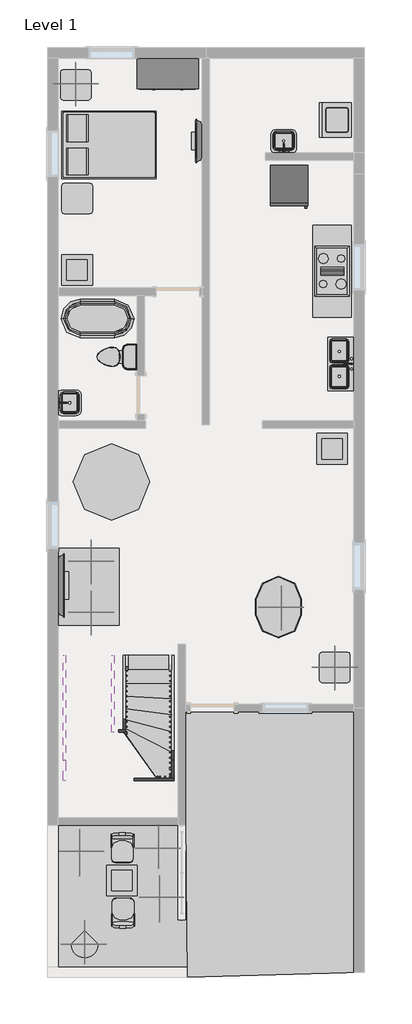
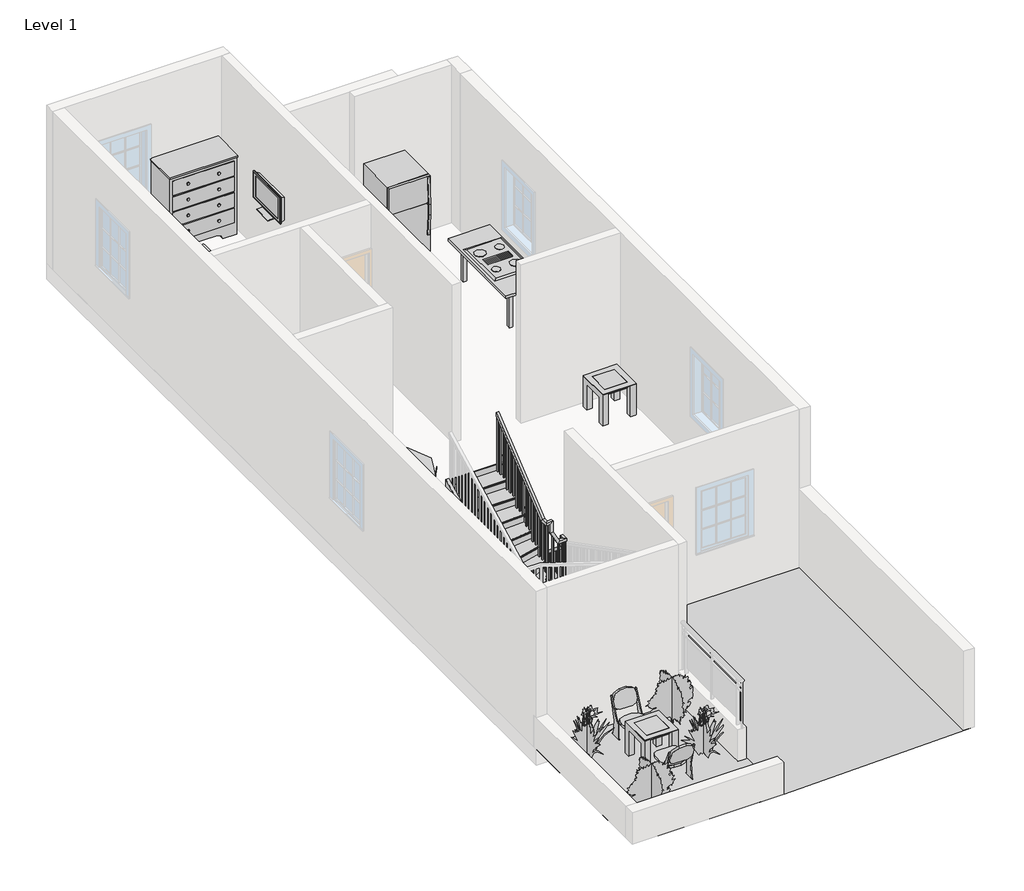
# One storey, part 3 of 3: 16 furniture elements, 9 geographic elements, 8 members, 7 flow terminals, 5 proxies, 1 railing, 1 stair flight.
"""IFC4 building model written with IfcOpenShell, lengths in millimetres."""

from ifc_helpers import new_model, si_unit, frame, origin, place, context, project, spatial, polyline, outline, extrude, faceted_brep, triangles, transform, mapped, element, save
from components import proxy_bb1e6e30, proxy_a13a33b2, proxy_718fa39f, flow_terminal_2b63360b, flow_terminal_a53be723, flow_terminal_62a433f7, toilet_domestic_3d_toilet_domestic_3d_f7549cf7, toilet_domestic_3d_toilet_domestic_3d_183bbd19, flow_terminal_db991eef, furniture_c8abb964, furniture_2babcf72, furniture_3d1d9cbc, furniture_56245f3a, furniture_fdf74506, furniture_b5c51a22, furniture_be1c6672, furniture_bbcc68ce, furniture_31d08a24, furniture_e8434c74, furniture_a5b052b6, rpc_plant_tropical_55f6ff97, rpc_plant_tropical_agave_1_5_93a2a214, rpc_plant_tropical_jungle_flame_3_9c4808c2, stair_flight_35bc4011

model = new_model("IFC4")

# Units and contexts
model_context = context("Model", 3, world=origin())
ifc_project = project(units=[si_unit("LENGTHUNIT", "METRE", prefix="MILLI")], contexts=[model_context])

# Site, building, storey
site = spatial("IfcSite", under=ifc_project)
building = spatial("IfcBuilding", under=site)
storey = spatial("IfcBuildingStorey", under=building, Name="Level 1", Elevation=0.0)

# Proxies
placement = place(None, origin())
element("IfcBuildingElementProxy", 1, Name="Building Element Proxy", at=placement, inside=storey, context=model_context, shape_type="Tessellation", body=[
    triangles([(-3017.7480675, -2501.1894814, 0.0), (-3017.7480675, -5523.7895782, 0.0), (-249.1479645, -5523.7895782, 0.0), (-274.5479585, -2501.1894814, 0.0)], [[1, 2, 4], [3, 4, 2]], closed=False),
])
element("IfcBuildingElementProxy", 2, Name="Building Element Proxy", at=placement, inside=storey, context=model_context, shape_type="Tessellation", body=[
    triangles([(-274.5479585, -240.5896025, 0.0), (3281.4520294, -240.5896025, 0.0), (3281.4520294, -5422.1893845, 0.0), (-249.1479645, -5523.7895782, 0.0), (-172.9479645, -138.9895994, 0.0)], [[1, 4, 3], [1, 2, 5], [2, 1, 3]], closed=False),
])
proxy_shape = proxy_bb1e6e30(model_context)
element("IfcBuildingElementProxy", 3, Name="Cook Top-4 Unit : 36\" x 20\"", ObjectType="Cook Top-4 Unit : 36\" x 20\"", at=placement, inside=storey, context=model_context, shape_type="MappedRepresentation", body=[
    mapped(proxy_shape, transform((2646.4520363, 8522.4104001, 0.0), x_axis=(0.0, -1.0, 0.0), y_axis=(1.0, 0.0, 0.0), z_axis=(0.0, 0.0, 1.0))),
])
proxy_2_shape = proxy_a13a33b2(model_context)
element("IfcBuildingElementProxy", 4, Name="Refrigerator : 30\" x 32\" RH", ObjectType="Refrigerator : 30\" x 32\" RH", at=placement, inside=storey, context=model_context, shape_type="MappedRepresentation", body=[
    mapped(proxy_2_shape, transform((1790.7895363, 10242.0614286, 0.0), x_axis=(1.0, 0.0, 0.0), y_axis=(0.0, 1.0, 0.0), z_axis=(0.0, 0.0, 1.0))),
])
proxy_3_shape = proxy_718fa39f(model_context)
element("IfcBuildingElementProxy", 5, Name="Washer : 27\" x 25\" x 35\"", ObjectType="Washer : 27\" x 25\" x 35\"", at=placement, inside=storey, context=model_context, shape_type="MappedRepresentation", body=[
    mapped(proxy_3_shape, transform((2989.1016011, 11111.8929316, 0.0), x_axis=(0.0, 1.0000000000000007, 0.0), y_axis=(-1.0000000000000007, 0.0, 0.0), z_axis=(0.0, 0.0, 1.0))),
])

# Flow terminals
flow_terminal_shape = flow_terminal_2b63360b(model_context)
element("IfcFlowTerminal", 6, ObjectType="Floor Drain - Rectangular : 5\"x5\" Strainer - 2\" Drain", at=placement, inside=storey, context=model_context, shape_type="MappedRepresentation", body=[
    mapped(flow_terminal_shape, transform((-2636.7479637, 7100.0104001, 0.0), x_axis=(1.0, 0.0, 0.0), y_axis=(0.0, 1.0, 0.0), z_axis=(0.0, 0.0, 1.0))),
])
element("IfcFlowTerminal", 7, ObjectType="Floor Drain - Rectangular : 5\"x5\" Strainer - 2\" Drain", at=placement, inside=storey, context=model_context, shape_type="MappedRepresentation", body=[
    mapped(flow_terminal_shape, transform((2849.6520363, 12205.4104001, 0.0), x_axis=(1.0, 0.0, 0.0), y_axis=(0.0, 1.0, 0.0), z_axis=(0.0, 0.0, 1.0))),
])
flow_terminal_2_shape = flow_terminal_a53be723(model_context)
element("IfcFlowTerminal", 8, ObjectType="Sink Kitchen-Double : 42\" x 21\"", at=placement, inside=storey, context=model_context, shape_type="MappedRepresentation", body=[
    mapped(flow_terminal_2_shape, transform((2821.9066352, 6696.5996407, 0.0), x_axis=(0.0, -1.0000000000000004, 0.0), y_axis=(1.0000000000000004, 0.0, 0.0), z_axis=(0.0, 0.0, 1.0))),
])
flow_terminal_3_shape = flow_terminal_62a433f7(model_context)
element("IfcFlowTerminal", 9, ObjectType="Sink Vanity-Square : 20\" x 18\"", at=placement, inside=storey, context=model_context, shape_type="MappedRepresentation", body=[
    mapped(flow_terminal_3_shape, transform((-2634.4025626, 5890.5211595, 0.0), x_axis=(0.0, 1.0000000000000002, 0.0), y_axis=(-1.0000000000000002, 0.0, 0.0), z_axis=(0.0, 0.0, 1.0))),
])
element("IfcFlowTerminal", 10, ObjectType="Sink Vanity-Square : 20\" x 18\"", at=placement, inside=storey, context=model_context, shape_type="MappedRepresentation", body=[
    mapped(flow_terminal_3_shape, transform((1696.9412769, 11064.7558012, 0.0), x_axis=(-1.0000000000000004, 0.0, 0.0), y_axis=(0.0, -1.0000000000000004, 0.0), z_axis=(0.0, 0.0, 1.0))),
])
toilet_domestic_3d_toilet_domestic_3d_shape = toilet_domestic_3d_toilet_domestic_3d_f7549cf7(model_context)
toilet_domestic_3d_toilet_domestic_3d_2_shape = toilet_domestic_3d_toilet_domestic_3d_183bbd19(model_context)
element("IfcFlowTerminal", 11, ObjectType="Toilet-Domestic-3D : Toilet-Domestic-3D", at=placement, inside=storey, context=model_context, shape_type="MappedRepresentation", body=[
    mapped(toilet_domestic_3d_toilet_domestic_3d_shape, transform((-1734.443991, 6820.6104001, 0.0), x_axis=(0.0, -1.0000000000000004, 0.0), y_axis=(1.0000000000000004, 0.0, 0.0), z_axis=(0.0, 0.0, 1.0))),
    mapped(toilet_domestic_3d_toilet_domestic_3d_2_shape, transform((-1734.443991, 6820.6104001, 0.0), x_axis=(0.0, -1.0000000000000004, 0.0), y_axis=(1.0000000000000004, 0.0, 0.0), z_axis=(0.0, 0.0, 1.0))),
])
flow_terminal_4_shape = flow_terminal_db991eef(model_context)
element("IfcFlowTerminal", 12, ObjectType="Tub-Free Standing-3D : 30\" x 60\"", at=placement, inside=storey, context=model_context, shape_type="MappedRepresentation", body=[
    mapped(flow_terminal_4_shape, transform((-2027.1479637, 7582.6104001, 0.0), x_axis=(0.0, 1.0000000000000002, 0.0), y_axis=(-1.0000000000000002, 0.0, 0.0), z_axis=(0.0, 0.0, 1.0))),
])

# Furniture
furniture_shape = furniture_c8abb964(model_context)
element("IfcFurniture", 13, ObjectType="Bed-Box : Double 53\" x 74\"", at=placement, inside=storey, context=model_context, shape_type="MappedRepresentation", body=[
    mapped(furniture_shape, transform((-2032.9774719, 10697.8579411, 0.0), x_axis=(0.0, 1.0, 0.0), y_axis=(-1.0, 0.0, 0.0), z_axis=(0.0, 0.0, 1.0))),
])
furniture_2_shape = furniture_2babcf72(model_context)
element("IfcFurniture", 14, ObjectType="Dresser : 48\" x 60\" x 24\"", at=placement, inside=storey, context=model_context, shape_type="MappedRepresentation", body=[
    mapped(furniture_2_shape, transform((-360.9547039, 12822.5733542, 0.0), x_axis=(1.0, 0.0, 0.0), y_axis=(0.0, 1.0, 0.0), z_axis=(0.0, 0.0, 1.0))),
])
furniture_3_shape = furniture_3d1d9cbc(model_context)
element("IfcFurniture", 15, ObjectType="Seating-Auditorium : 18\" x 24\" x 30\"", at=placement, inside=storey, context=model_context, shape_type="MappedRepresentation", body=[
    mapped(furniture_3_shape, transform((-1371.1200948, -2743.1141901, 0.0), x_axis=(-1.0000000000000004, 0.0, 0.0), y_axis=(0.0, -1.0000000000000004, 0.0), z_axis=(0.0, 0.0, 1.0))),
])
element("IfcFurniture", 16, ObjectType="Seating-Auditorium : 18\" x 24\" x 30\"", at=placement, inside=storey, context=model_context, shape_type="MappedRepresentation", body=[
    mapped(furniture_3_shape, transform((-1679.8758325, -4443.6650097, 0.0), x_axis=(1.0, 0.0, 0.0), y_axis=(0.0, 1.0, 0.0), z_axis=(0.0, 0.0, 1.0))),
])
furniture_4_shape = furniture_56245f3a(model_context)
element("IfcFurniture", 17, ObjectType="TV - Flat Screen : 32\"", at=placement, inside=storey, context=model_context, shape_type="MappedRepresentation", body=[
    mapped(furniture_4_shape, transform((-2.8865873, 11109.265886, 1041.4), x_axis=(0.0, -1.0000000000000002, 0.0), y_axis=(1.0000000000000002, 0.0, 0.0), z_axis=(0.0, 0.0, 1.0))),
])
furniture_5_shape = furniture_fdf74506(model_context)
element("IfcFurniture", 18, ObjectType="TV - Flat Screen : 50\"", at=placement, inside=storey, context=model_context, shape_type="MappedRepresentation", body=[
    mapped(furniture_5_shape, transform((-2756.00934, 2277.9549142, 1041.4), x_axis=(0.0, 1.0000000000000002, 0.0), y_axis=(-1.0000000000000002, 0.0, 0.0), z_axis=(0.0, 0.0, 1.0))),
])
furniture_6_shape = furniture_b5c51a22(model_context)
element("IfcFurniture", 19, ObjectType="Table-Coffee : 24\" x 24\" x 24\"", at=placement, inside=storey, context=model_context, shape_type="MappedRepresentation", body=[
    mapped(furniture_6_shape, transform((-2451.8137304, 8452.5993223, 0.0), x_axis=(1.0, 0.0, 0.0), y_axis=(0.0, 1.0, 0.0), z_axis=(0.0, 0.0, 1.0))),
])
element("IfcFurniture", 20, ObjectType="Table-Coffee : 24\" x 24\" x 24\"", at=placement, inside=storey, context=model_context, shape_type="MappedRepresentation", body=[
    mapped(furniture_6_shape, transform((2628.1862696, 4896.5993223, 0.0), x_axis=(1.0, 0.0, 0.0), y_axis=(0.0, 1.0, 0.0), z_axis=(0.0, 0.0, 1.0))),
])
element("IfcFurniture", 21, ObjectType="Table-Coffee : 24\" x 24\" x 24\"", at=placement, inside=storey, context=model_context, shape_type="MappedRepresentation", body=[
    mapped(furniture_6_shape, transform((-1562.8137304, -3688.6006777, 0.0), x_axis=(1.0, 0.0, 0.0), y_axis=(0.0, 1.0, 0.0), z_axis=(0.0, 0.0, 1.0))),
])
furniture_7_shape = furniture_be1c6672(model_context)
element("IfcFurniture", 22, ObjectType="Table-Dining Oval : 36\" x 48\"", at=placement, inside=storey, context=model_context, shape_type="MappedRepresentation", body=[
    mapped(furniture_7_shape, transform((1221.5536757, 2244.0300722, 0.0), x_axis=(0.0, 1.0000000000000002, 0.0), y_axis=(-1.0000000000000002, 0.0, 0.0), z_axis=(0.0, 0.0, 1.0))),
])
furniture_8_shape = furniture_bbcc68ce(model_context)
element("IfcFurniture", 23, ObjectType="Table-Dining Round w Chairs : 60\" Diameter", at=placement, inside=storey, context=model_context, shape_type="MappedRepresentation", body=[
    mapped(furniture_8_shape, transform((-1851.4299309, 4516.2890886, 0.0), x_axis=(1.0, 0.0, 0.0), y_axis=(0.0, 1.0, 0.0), z_axis=(0.0, 0.0, 1.0))),
])
furniture_9_shape = furniture_31d08a24(model_context)
element("IfcFurniture", 24, ObjectType="Table-End : 24\" x 24\"", at=placement, inside=storey, context=model_context, shape_type="MappedRepresentation", body=[
    mapped(furniture_9_shape, transform((-2767.481594, 12078.4104001, 0.0), x_axis=(1.0, 0.0, 0.0), y_axis=(0.0, 1.0, 0.0), z_axis=(0.0, 0.0, 1.0))),
])
element("IfcFurniture", 25, ObjectType="Table-End : 24\" x 24\"", at=placement, inside=storey, context=model_context, shape_type="MappedRepresentation", body=[
    mapped(furniture_9_shape, transform((-2742.081594, 9817.8104001, 0.0), x_axis=(1.0, 0.0, 0.0), y_axis=(0.0, 1.0, 0.0), z_axis=(0.0, 0.0, 1.0))),
])
element("IfcFurniture", 26, ObjectType="Table-End : 24\" x 24\"", at=placement, inside=storey, context=model_context, shape_type="MappedRepresentation", body=[
    mapped(furniture_9_shape, transform((2388.718406, 492.2787082, 0.0), x_axis=(1.0, 0.0, 0.0), y_axis=(0.0, 1.0, 0.0), z_axis=(0.0, 0.0, 1.0))),
])
furniture_10_shape = furniture_e8434c74(model_context)
element("IfcFurniture", 27, ObjectType="Table-Rectangular : 60\" x 48\"", at=placement, inside=storey, context=model_context, shape_type="MappedRepresentation", body=[
    mapped(furniture_10_shape, transform((-2204.9479637, 2248.6104001, 0.0), x_axis=(0.0, 1.0, 0.0), y_axis=(-1.0, 0.0, 0.0), z_axis=(0.0, 0.0, 1.0))),
])
furniture_11_shape = furniture_a5b052b6(model_context)
element("IfcFurniture", 28, ObjectType="Table-Rectangular : 72\" x 30\"", at=placement, inside=storey, context=model_context, shape_type="MappedRepresentation", body=[
    mapped(furniture_11_shape, transform((2646.4520363, 8522.4104001, 0.0), x_axis=(0.0, 1.0, 0.0), y_axis=(-1.0, 0.0, 0.0), z_axis=(0.0, 0.0, 1.0))),
])

# Geographic elements
rpc_plant_tropical_shape = rpc_plant_tropical_55f6ff97(model_context)
element("IfcGeographicElement", 29, ObjectType="RPC Plant - Tropical", at=placement, inside=storey, context=model_context, shape_type="MappedRepresentation", body=[
    mapped(rpc_plant_tropical_shape, transform((-2382.7479637, -3009.1895999, 0.0), x_axis=(1.0, 0.0, 0.0), y_axis=(0.0, 1.0, 0.0), z_axis=(0.0, 0.0, 1.0))),
])
element("IfcGeographicElement", 30, ObjectType="RPC Plant - Tropical", at=placement, inside=storey, context=model_context, shape_type="MappedRepresentation", body=[
    mapped(rpc_plant_tropical_shape, transform((-788.8979637, -3923.5895999, 0.0), x_axis=(1.0, 0.0, 0.0), y_axis=(0.0, 1.0, 0.0), z_axis=(0.0, 0.0, 1.0))),
])
rpc_plant_tropical_agave_1_5_shape = rpc_plant_tropical_agave_1_5_93a2a214(model_context)
element("IfcGeographicElement", 31, ObjectType="RPC Plant - Tropical : Agave - 1.5'", at=placement, inside=storey, context=model_context, shape_type="MappedRepresentation", body=[
    mapped(rpc_plant_tropical_agave_1_5_shape, transform((-2458.9479637, 12256.2104001, 609.6), x_axis=(1.0, 0.0, 0.0), y_axis=(0.0, 1.0, 0.0), z_axis=(0.0, 0.0, 1.0))),
])
element("IfcGeographicElement", 32, ObjectType="RPC Plant - Tropical : Agave - 1.5'", at=placement, inside=storey, context=model_context, shape_type="MappedRepresentation", body=[
    mapped(rpc_plant_tropical_agave_1_5_shape, transform((2697.2520363, 644.6787082, 609.6), x_axis=(1.0, 0.0, 0.0), y_axis=(0.0, 1.0, 0.0), z_axis=(0.0, 0.0, 1.0))),
])
element("IfcGeographicElement", 33, ObjectType="RPC Plant - Tropical : Agave - 1.5'", at=placement, inside=storey, context=model_context, shape_type="MappedRepresentation", body=[
    mapped(rpc_plant_tropical_agave_1_5_shape, transform((1630.4520363, 1842.2104001, 609.6), x_axis=(1.0, 0.0, 0.0), y_axis=(0.0, 1.0, 0.0), z_axis=(0.0, 0.0, 1.0))),
])
element("IfcGeographicElement", 34, ObjectType="RPC Plant - Tropical : Agave - 1.5'", at=placement, inside=storey, context=model_context, shape_type="MappedRepresentation", body=[
    mapped(rpc_plant_tropical_agave_1_5_shape, transform((-2154.1479637, 2756.6104001, 660.4), x_axis=(1.0, 0.0, 0.0), y_axis=(0.0, 1.0, 0.0), z_axis=(0.0, 0.0, 1.0))),
])
element("IfcGeographicElement", 35, ObjectType="RPC Plant - Tropical : Agave - 1.5'", at=placement, inside=storey, context=model_context, shape_type="MappedRepresentation", body=[
    mapped(rpc_plant_tropical_agave_1_5_shape, transform((-2154.1479637, 1740.6104001, 660.4), x_axis=(1.0, 0.0, 0.0), y_axis=(0.0, 1.0, 0.0), z_axis=(0.0, 0.0, 1.0))),
])
rpc_plant_tropical_jungle_flame_3_shape = rpc_plant_tropical_jungle_flame_3_9c4808c2(model_context)
element("IfcGeographicElement", 36, ObjectType="RPC Plant - Tropical : Jungle Flame - 3'", at=placement, inside=storey, context=model_context, shape_type="MappedRepresentation", body=[
    mapped(rpc_plant_tropical_jungle_flame_3_shape, transform((-2281.1479637, -4863.3895999, 0.0), x_axis=(1.0, 0.0, 0.0), y_axis=(0.0, 1.0, 0.0), z_axis=(0.0, 0.0, 1.0))),
])
element("IfcGeographicElement", 37, ObjectType="RPC Plant - Tropical : Jungle Flame - 3'", at=placement, inside=storey, context=model_context, shape_type="MappedRepresentation", body=[
    mapped(rpc_plant_tropical_jungle_flame_3_shape, transform((-807.9479637, -2958.3895999, 0.0), x_axis=(1.0, 0.0, 0.0), y_axis=(0.0, 1.0, 0.0), z_axis=(0.0, 0.0, 1.0))),
])

# Members
element("IfcMember", 38, ObjectType="Stringer - 2\" Width", at=placement, inside=storey, context=model_context, shape_type="SweptSolid", body=[
    extrude(outline(polyline([(880.742092, 229.639954), (880.742092, 0.0), (660.9797744, 0.0), (-1206.6750997, 962.500629), (-1206.6750997, 1305.3956453), (880.742092, 229.639954)])), frame((-553.9479637, 0.0, 0.0), z_axis=(1.0, 0.0, 0.0), x_axis=(0.0, 1.0, 0.0)), (0.0, 0.0, 1.0), 50.8),
])
element("IfcMember", 39, ObjectType="Stringer - 2\" Width", at=placement, inside=storey, context=model_context, shape_type="SweptSolid", body=[
    extrude(outline(polyline([(-553.9479637, -1206.6750997), (-503.1479637, -1206.6750997), (-503.1479637, -1561.3895999), (-553.9479637, -1561.3895999), (-553.9479637, -1206.6750997)])), frame((0.0, 0.0, 962.500629), z_axis=(0.0, 0.0, 1.0), x_axis=(1.0, 0.0, 0.0)), (0.0, 0.0, 1.0), 342.8950162),
])
element("IfcMember", 40, ObjectType="Stringer - 2\" Width", at=placement, inside=storey, context=model_context, shape_type="SweptSolid", body=[
    extrude(outline(polyline([(1000.5956453, -503.1479637), (1289.0952212, -503.1479637), (1969.9972697, -2625.1678464), (1969.9972697, -2662.1479637), (1638.9682298, -2662.1479637), (1000.5956453, -672.6704467), (1000.5956453, -503.1479637)])), frame((0.0, -1612.1895999, 0.0), z_axis=(0.0, 1.0, 0.0), x_axis=(0.0, 0.0, 1.0)), (0.0, 0.0, 1.0), 50.8),
])
element("IfcMember", 41, ObjectType="Stringer - 2\" Width", at=placement, inside=storey, context=model_context, shape_type="SweptSolid", body=[
    extrude(outline(polyline([(-2662.1479637, -1612.1895999), (-2712.9479637, -1612.1895999), (-2712.9479637, -1206.6750997), (-2662.1479637, -1206.6750997), (-2662.1479637, -1612.1895999)])), frame((0.0, 0.0, 1649.8904473), z_axis=(0.0, 0.0, 1.0), x_axis=(1.0, 0.0, 0.0)), (0.0, 0.0, 1.0), 320.1068224),
])
element("IfcMember", 42, ObjectType="Stringer - 2\" Width", at=placement, inside=storey, context=model_context, shape_type="SweptSolid", body=[
    extrude(outline(polyline([(-1206.6750997, 1649.8904473), (-1206.6750997, 1969.9972697), (880.742092, 3045.7529609), (880.742092, 2725.6461385), (-1206.6750997, 1649.8904473)])), frame((-2712.9479637, 0.0, 0.0), z_axis=(1.0, 0.0, 0.0), x_axis=(0.0, 1.0, 0.0)), (0.0, 0.0, 1.0), 50.8),
])
element("IfcMember", 43, ObjectType="Stringer - 2\" Width", at=placement, inside=storey, context=model_context, shape_type="SweptSolid", body=[
    extrude(outline(polyline([(880.742092, 176.1764461), (880.742092, 0.0), (614.4804474, 0.0), (-596.1895999, 987.1410923), (-596.1895999, 1380.418648), (880.742092, 176.1764461)])), frame((-1519.1479637, 0.0, 0.0), z_axis=(1.0, 0.0, 0.0), x_axis=(0.0, 1.0, 0.0)), (0.0, 0.0, 1.0), 50.8),
])
element("IfcMember", 44, ObjectType="Stringer - 2\" Width", at=placement, inside=storey, context=model_context, shape_type="SweptSolid", body=[
    extrude(outline(polyline([(1028.5617647, -1468.3479637), (1573.2682978, -1468.3479637), (1926.1409689, -1674.9850811), (1926.1409689, -1696.9479637), (1360.465107, -1696.9479637), (1028.5617647, -1502.590181), (1028.5617647, -1468.3479637)])), frame((0.0, -646.9895999, 0.0), z_axis=(0.0, 1.0, 0.0), x_axis=(0.0, 0.0, 1.0)), (0.0, 0.0, 1.0), 50.8),
])
element("IfcMember", 45, ObjectType="Stringer - 2\" Width", at=placement, inside=storey, context=model_context, shape_type="SweptSolid", body=[
    extrude(outline(polyline([(-646.9895999, 1532.8634131), (-646.9895999, 1926.1409689), (880.742092, 3171.8038432), (880.742092, 2778.5262875), (-646.9895999, 1532.8634131)])), frame((-1747.7479637, 0.0, 0.0), z_axis=(1.0, 0.0, 0.0), x_axis=(0.0, 1.0, 0.0)), (0.0, 0.0, 1.0), 50.8),
])

# Railing
element("IfcRailing", 46, ObjectType="Handrail - Rectangular", at=placement, inside=storey, context=model_context, shape_type="SolidModel", body=[
    faceted_brep([(-1417.5479637, 880.742092, 1025.2529681), (-1417.5479637, 880.742092, 959.7067088), (-1468.3479637, 880.742092, 959.7067088), (-1468.3479637, 880.742092, 1025.2529681), (-1417.5479637, -570.7895999, 2208.7848338), (-1417.5479637, -621.5895999, 2184.659247), (-1468.3479637, -621.5895999, 2184.659247), (-1468.3479637, -570.7895999, 2208.7848338), (-1417.5479637, -570.7895999, 2414.6281882), (-1417.5479637, -621.5895999, 2363.8281882), (-1468.3479637, -621.5895999, 2363.8281882), (-1468.3479637, -570.7895999, 2414.6281882), (-1417.5479637, -697.7895999, 2414.6281882), (-1417.5479637, -697.7895999, 2363.8281882), (-1468.3479637, -646.9895999, 2363.8281882), (-1468.3479637, -646.9895999, 2414.6281882), (-1544.5479637, -697.7895999, 2414.6281882), (-1573.6692975, -697.7895999, 2363.8281882), (-1573.6692975, -646.9895999, 2363.8281882), (-1544.5479637, -646.9895999, 2414.6281882), (-1671.5479637, -697.7895999, 2631.5051451), (-1722.3479637, -697.7895999, 2617.7256424), (-1722.3479637, -646.9895999, 2617.7256424), (-1671.5479637, -646.9895999, 2631.5051451), (-1671.5479637, -697.7895999, 2837.3484995), (-1722.3479637, -697.7895999, 2786.5484995), (-1722.3479637, -646.9895999, 2786.5484995), (-1671.5479637, -646.9895999, 2837.3484995), (-1798.5479637, -697.7895999, 2837.3484995), (-1798.5479637, -697.7895999, 2786.5484995), (-1747.7479637, -646.9895999, 2786.5484995), (-1747.7479637, -646.9895999, 2837.3484995), (-1798.5479637, -570.7895999, 2837.3484995), (-1798.5479637, -552.7041868, 2786.5484995), (-1747.7479637, -552.7041868, 2786.5484995), (-1747.7479637, -570.7895999, 2837.3484995), (-1798.5479637, 880.742092, 4020.8803652), (-1747.7479637, 880.742092, 4020.8803652), (-1747.7479637, 880.742092, 3955.3341059), (-1798.5479637, 880.742092, 3955.3341059)], [[[0, 1, 2, 3]], [[1, 0, 4, 5]], [[2, 1, 5, 6]], [[3, 2, 6, 7]], [[0, 3, 7, 4]], [[5, 4, 8, 9]], [[6, 5, 9, 10]], [[7, 6, 10, 11]], [[4, 7, 11, 8]], [[9, 8, 12, 13]], [[10, 9, 13, 14]], [[11, 10, 14, 15]], [[8, 11, 15, 12]], [[13, 12, 16, 17]], [[14, 13, 17, 18]], [[15, 14, 18, 19]], [[12, 15, 19, 16]], [[17, 16, 20, 21]], [[18, 17, 21, 22]], [[19, 18, 22, 23]], [[16, 19, 23, 20]], [[21, 20, 24, 25]], [[22, 21, 25, 26]], [[23, 22, 26, 27]], [[20, 23, 27, 24]], [[25, 24, 28, 29]], [[26, 25, 29, 30]], [[27, 26, 30, 31]], [[24, 27, 31, 28]], [[29, 28, 32, 33]], [[30, 29, 33, 34]], [[31, 30, 34, 35]], [[28, 31, 35, 32]], [[36, 37, 38, 39]], [[33, 32, 36, 39]], [[34, 33, 39, 38]], [[35, 34, 38, 37]], [[32, 35, 37, 36]]]),
    extrude(outline(polyline([(771.4527565, 3866.2231262), (790.5027565, 3881.7558784), (790.5027565, 2878.6666667), (771.4527565, 2878.6666667), (771.4527565, 3866.2231262)])), frame((-1782.6729637, 0.0, 0.0), z_axis=(1.0, 0.0, 0.0), x_axis=(0.0, 1.0, 0.0)), (0.0, 0.0, 1.0), 19.05),
    extrude(outline(polyline([(669.8527565, 3783.3817813), (688.9027565, 3798.9145334), (688.9027565, 2878.6666667), (669.8527565, 2878.6666667), (669.8527565, 3783.3817813)])), frame((-1782.6729637, 0.0, 0.0), z_axis=(1.0, 0.0, 0.0), x_axis=(0.0, 1.0, 0.0)), (0.0, 0.0, 1.0), 19.05),
    extrude(outline(polyline([(568.2527565, 3700.5404364), (587.3027565, 3716.0731885), (587.3027565, 2709.3333333), (568.2527565, 2709.3333333), (568.2527565, 3700.5404364)])), frame((-1782.6729637, 0.0, 0.0), z_axis=(1.0, 0.0, 0.0), x_axis=(0.0, 1.0, 0.0)), (0.0, 0.0, 1.0), 19.05),
    extrude(outline(polyline([(466.6527565, 3617.6990914), (485.7027565, 3633.2318436), (485.7027565, 2709.3333333), (466.6527565, 2709.3333333), (466.6527565, 3617.6990914)])), frame((-1782.6729637, 0.0, 0.0), z_axis=(1.0, 0.0, 0.0), x_axis=(0.0, 1.0, 0.0)), (0.0, 0.0, 1.0), 19.05),
    extrude(outline(polyline([(365.0527565, 3534.8577465), (384.1027565, 3550.3904987), (384.1027565, 2709.3333333), (365.0527565, 2709.3333333), (365.0527565, 3534.8577465)])), frame((-1782.6729637, 0.0, 0.0), z_axis=(1.0, 0.0, 0.0), x_axis=(0.0, 1.0, 0.0)), (0.0, 0.0, 1.0), 19.05),
    extrude(outline(polyline([(263.4527565, 3452.0164016), (282.5027565, 3467.5491538), (282.5027565, 2540.0), (263.4527565, 2540.0), (263.4527565, 3452.0164016)])), frame((-1782.6729637, 0.0, 0.0), z_axis=(1.0, 0.0, 0.0), x_axis=(0.0, 1.0, 0.0)), (0.0, 0.0, 1.0), 19.05),
    extrude(outline(polyline([(161.8527565, 3369.1750567), (180.9027565, 3384.7078088), (180.9027565, 2540.0), (161.8527565, 2540.0), (161.8527565, 3369.1750567)])), frame((-1782.6729637, 0.0, 0.0), z_axis=(1.0, 0.0, 0.0), x_axis=(0.0, 1.0, 0.0)), (0.0, 0.0, 1.0), 19.05),
    extrude(outline(polyline([(60.2527565, 3286.3337117), (79.3027565, 3301.8664639), (79.3027565, 2540.0), (60.2527565, 2540.0), (60.2527565, 3286.3337117)])), frame((-1782.6729637, 0.0, 0.0), z_axis=(1.0, 0.0, 0.0), x_axis=(0.0, 1.0, 0.0)), (0.0, 0.0, 1.0), 19.05),
    extrude(outline(polyline([(-41.3472435, 3203.4923668), (-22.2972435, 3219.025119), (-22.2972435, 2370.6666667), (-41.3472435, 2370.6666667), (-41.3472435, 3203.4923668)])), frame((-1782.6729637, 0.0, 0.0), z_axis=(1.0, 0.0, 0.0), x_axis=(0.0, 1.0, 0.0)), (0.0, 0.0, 1.0), 19.05),
    extrude(outline(polyline([(-142.9472435, 3120.6510219), (-123.8972435, 3136.1837741), (-123.8972435, 2370.6666667), (-142.9472435, 2370.6666667), (-142.9472435, 3120.6510219)])), frame((-1782.6729637, 0.0, 0.0), z_axis=(1.0, 0.0, 0.0), x_axis=(0.0, 1.0, 0.0)), (0.0, 0.0, 1.0), 19.05),
    extrude(outline(polyline([(-244.5472435, 3037.809677), (-225.4972435, 3053.3424291), (-225.4972435, 2201.3333333), (-244.5472435, 2201.3333333), (-244.5472435, 3037.809677)])), frame((-1782.6729637, 0.0, 0.0), z_axis=(1.0, 0.0, 0.0), x_axis=(0.0, 1.0, 0.0)), (0.0, 0.0, 1.0), 19.05),
    extrude(outline(polyline([(-346.1472435, 2954.9683321), (-327.0972435, 2970.5010842), (-327.0972435, 2201.3333333), (-346.1472435, 2201.3333333), (-346.1472435, 2954.9683321)])), frame((-1782.6729637, 0.0, 0.0), z_axis=(1.0, 0.0, 0.0), x_axis=(0.0, 1.0, 0.0)), (0.0, 0.0, 1.0), 19.05),
    extrude(outline(polyline([(-447.7472435, 2872.1269871), (-428.6972435, 2887.6597393), (-428.6972435, 2032.0), (-447.7472435, 2032.0), (-447.7472435, 2872.1269871)])), frame((-1782.6729637, 0.0, 0.0), z_axis=(1.0, 0.0, 0.0), x_axis=(0.0, 1.0, 0.0)), (0.0, 0.0, 1.0), 19.05),
    extrude(outline(polyline([(-549.3472435, 2789.2856422), (-530.2972435, 2804.8183944), (-530.2972435, 2032.0), (-549.3472435, 2032.0), (-549.3472435, 2789.2856422)])), frame((-1782.6729637, 0.0, 0.0), z_axis=(1.0, 0.0, 0.0), x_axis=(0.0, 1.0, 0.0)), (0.0, 0.0, 1.0), 19.05),
    extrude(outline(polyline([(2496.5834745, -1651.4088674), (2529.115018, -1670.4588674), (1524.0, -1670.4588674), (1524.0, -1651.4088674), (2496.5834745, -1651.4088674)])), frame((0.0, -681.9145999, 0.0), z_axis=(0.0, 1.0, 0.0), x_axis=(0.0, 0.0, 1.0)), (0.0, 0.0, 1.0), 19.05),
    extrude(outline(polyline([(2323.0819089, -1549.8088674), (2355.6134525, -1568.8588674), (1524.0, -1568.8588674), (1524.0, -1549.8088674), (2323.0819089, -1549.8088674)])), frame((0.0, -681.9145999, 0.0), z_axis=(0.0, 1.0, 0.0), x_axis=(0.0, 0.0, 1.0)), (0.0, 0.0, 1.0), 19.05),
    extrude(outline(polyline([(-551.182908, 2127.2519138), (-532.132908, 2111.7191617), (-532.132908, 1016.0), (-551.182908, 1016.0), (-551.182908, 2127.2519138)])), frame((-1452.4729637, 0.0, 0.0), z_axis=(1.0, 0.0, 0.0), x_axis=(0.0, 1.0, 0.0)), (0.0, 0.0, 1.0), 19.05),
    extrude(outline(polyline([(-449.582908, 2044.4105689), (-430.532908, 2028.8778167), (-430.532908, 1016.0), (-449.582908, 1016.0), (-449.582908, 2044.4105689)])), frame((-1452.4729637, 0.0, 0.0), z_axis=(1.0, 0.0, 0.0), x_axis=(0.0, 1.0, 0.0)), (0.0, 0.0, 1.0), 19.05),
    extrude(outline(polyline([(-347.982908, 1961.569224), (-328.932908, 1946.0364718), (-328.932908, 846.6666667), (-347.982908, 846.6666667), (-347.982908, 1961.569224)])), frame((-1452.4729637, 0.0, 0.0), z_axis=(1.0, 0.0, 0.0), x_axis=(0.0, 1.0, 0.0)), (0.0, 0.0, 1.0), 19.05),
    extrude(outline(polyline([(-246.382908, 1878.7278791), (-227.332908, 1863.1951269), (-227.332908, 846.6666667), (-246.382908, 846.6666667), (-246.382908, 1878.7278791)])), frame((-1452.4729637, 0.0, 0.0), z_axis=(1.0, 0.0, 0.0), x_axis=(0.0, 1.0, 0.0)), (0.0, 0.0, 1.0), 19.05),
    extrude(outline(polyline([(-144.782908, 1795.8865341), (-125.732908, 1780.353782), (-125.732908, 677.3333333), (-144.782908, 677.3333333), (-144.782908, 1795.8865341)])), frame((-1452.4729637, 0.0, 0.0), z_axis=(1.0, 0.0, 0.0), x_axis=(0.0, 1.0, 0.0)), (0.0, 0.0, 1.0), 19.05),
    extrude(outline(polyline([(-43.182908, 1713.0451892), (-24.132908, 1697.5124371), (-24.132908, 677.3333333), (-43.182908, 677.3333333), (-43.182908, 1713.0451892)])), frame((-1452.4729637, 0.0, 0.0), z_axis=(1.0, 0.0, 0.0), x_axis=(0.0, 1.0, 0.0)), (0.0, 0.0, 1.0), 19.05),
    extrude(outline(polyline([(58.417092, 1630.2038443), (77.467092, 1614.6710921), (77.467092, 508.0), (58.417092, 508.0), (58.417092, 1630.2038443)])), frame((-1452.4729637, 0.0, 0.0), z_axis=(1.0, 0.0, 0.0), x_axis=(0.0, 1.0, 0.0)), (0.0, 0.0, 1.0), 19.05),
    extrude(outline(polyline([(160.017092, 1547.3624994), (179.067092, 1531.8297472), (179.067092, 508.0), (160.017092, 508.0), (160.017092, 1547.3624994)])), frame((-1452.4729637, 0.0, 0.0), z_axis=(1.0, 0.0, 0.0), x_axis=(0.0, 1.0, 0.0)), (0.0, 0.0, 1.0), 19.05),
    extrude(outline(polyline([(261.617092, 1464.5211545), (280.667092, 1448.9884023), (280.667092, 508.0), (261.617092, 508.0), (261.617092, 1464.5211545)])), frame((-1452.4729637, 0.0, 0.0), z_axis=(1.0, 0.0, 0.0), x_axis=(0.0, 1.0, 0.0)), (0.0, 0.0, 1.0), 19.05),
    extrude(outline(polyline([(363.217092, 1381.6798095), (382.267092, 1366.1470574), (382.267092, 338.6666667), (363.217092, 338.6666667), (363.217092, 1381.6798095)])), frame((-1452.4729637, 0.0, 0.0), z_axis=(1.0, 0.0, 0.0), x_axis=(0.0, 1.0, 0.0)), (0.0, 0.0, 1.0), 19.05),
    extrude(outline(polyline([(464.817092, 1298.8384646), (483.867092, 1283.3057124), (483.867092, 338.6666667), (464.817092, 338.6666667), (464.817092, 1298.8384646)])), frame((-1452.4729637, 0.0, 0.0), z_axis=(1.0, 0.0, 0.0), x_axis=(0.0, 1.0, 0.0)), (0.0, 0.0, 1.0), 19.05),
    extrude(outline(polyline([(566.417092, 1215.9971197), (585.467092, 1200.4643675), (585.467092, 338.6666667), (566.417092, 338.6666667), (566.417092, 1215.9971197)])), frame((-1452.4729637, 0.0, 0.0), z_axis=(1.0, 0.0, 0.0), x_axis=(0.0, 1.0, 0.0)), (0.0, 0.0, 1.0), 19.05),
    extrude(outline(polyline([(668.017092, 1133.1557748), (687.067092, 1117.6230226), (687.067092, 169.3333333), (668.017092, 169.3333333), (668.017092, 1133.1557748)])), frame((-1452.4729637, 0.0, 0.0), z_axis=(1.0, 0.0, 0.0), x_axis=(0.0, 1.0, 0.0)), (0.0, 0.0, 1.0), 19.05),
    extrude(outline(polyline([(769.617092, 1050.3144298), (788.667092, 1034.7816777), (788.667092, 169.3333333), (769.617092, 169.3333333), (769.617092, 1050.3144298)])), frame((-1452.4729637, 0.0, 0.0), z_axis=(1.0, 0.0, 0.0), x_axis=(0.0, 1.0, 0.0)), (0.0, 0.0, 1.0), 19.05),
    extrude(outline(polyline([(-1763.6229637, -650.9472435), (-1782.6729637, -650.9472435), (-1782.6729637, -631.8972435), (-1763.6229637, -631.8972435), (-1763.6229637, -650.9472435)])), frame((0.0, 0.0, 1862.6666667), z_axis=(0.0, 0.0, 1.0), x_axis=(1.0, 0.0, 0.0)), (0.0, 0.0, 1.0), 923.8818329),
    extrude(outline(polyline([(-1763.6229637, -662.8645999), (-1763.6229637, -681.9145999), (-1782.6729637, -681.9145999), (-1782.6729637, -662.8645999), (-1763.6229637, -662.8645999)])), frame((0.0, 0.0, 1862.6666667), z_axis=(0.0, 0.0, 1.0), x_axis=(1.0, 0.0, 0.0)), (0.0, 0.0, 1.0), 923.8818329),
    extrude(outline(polyline([(-1748.8370599, -662.8645999), (-1748.8370599, -681.9145999), (-1767.8870599, -681.9145999), (-1767.8870599, -662.8645999), (-1748.8370599, -662.8645999)])), frame((0.0, 0.0, 1693.3333333), z_axis=(0.0, 0.0, 1.0), x_axis=(1.0, 0.0, 0.0)), (0.0, 0.0, 1.0), 1093.2151662),
    extrude(outline(polyline([(-1448.2088674, -662.8645999), (-1448.2088674, -681.9145999), (-1467.2588674, -681.9145999), (-1467.2588674, -662.8645999), (-1448.2088674, -662.8645999)])), frame((0.0, 0.0, 1354.6666667), z_axis=(0.0, 0.0, 1.0), x_axis=(1.0, 0.0, 0.0)), (0.0, 0.0, 1.0), 1009.1615215),
    extrude(outline(polyline([(-1452.4729637, -662.8645999), (-1433.4229637, -662.8645999), (-1433.4229637, -681.9145999), (-1452.4729637, -681.9145999), (-1452.4729637, -662.8645999)])), frame((0.0, 0.0, 1185.3333333), z_axis=(0.0, 0.0, 1.0), x_axis=(1.0, 0.0, 0.0)), (0.0, 0.0, 1.0), 1178.4948549),
    extrude(outline(polyline([(-1452.4729637, -631.8972435), (-1433.4229637, -631.8972435), (-1433.4229637, -650.9472435), (-1452.4729637, -650.9472435), (-1452.4729637, -631.8972435)])), frame((0.0, 0.0, 1185.3333333), z_axis=(0.0, 0.0, 1.0), x_axis=(1.0, 0.0, 0.0)), (0.0, 0.0, 1.0), 1178.4948549),
    extrude(outline(polyline([(861.692092, 3939.8013537), (880.742092, 3955.3341059), (880.742092, 2878.6666667), (861.692092, 2878.6666667), (861.692092, 3939.8013537)])), frame((-1782.6729637, 0.0, 0.0), z_axis=(1.0, 0.0, 0.0), x_axis=(0.0, 1.0, 0.0)), (0.0, 0.0, 1.0), 19.05),
    extrude(outline(polyline([(861.692092, 975.239461), (880.742092, 959.7067088), (880.742092, 169.3333333), (861.692092, 169.3333333), (861.692092, 975.239461)])), frame((-1452.4729637, 0.0, 0.0), z_axis=(1.0, 0.0, 0.0), x_axis=(0.0, 1.0, 0.0)), (0.0, 0.0, 1.0), 19.05),
])

# Stair flight
stair_flight_shape = stair_flight_35bc4011(model_context)
element("IfcStairFlight", 47, ObjectType="2\" Tread 1\" Nosing 1/4\" Riser", at=placement, inside=storey, context=model_context, shape_type="MappedRepresentation", body=[
    mapped(stair_flight_shape, transform((0.0, 0.0, 0.0), x_axis=(1.0, 0.0, 0.0), y_axis=(0.0, 1.0, 0.0), z_axis=(0.0, 0.0, 1.0))),
])

save(model, "model.ifc")

# Revit data of these elements
# Type "Cook Top-4 Unit : 36\" x 20\""
#   Assembly Code = "E1090400"
#   Depth = 2' - 0"
#   Width = 3' - 0"
#   Burner Material = Steel, Chrome Plated
#   Cooktop Material = Steel, Polished
#   Default Elevation = 0
# Type "Refrigerator : 30\" x 32\" RH"
#   Label = "REF."
#   Assembly Code = "E1090400"
#   Depth = 2' - 7 3/4"
#   Handle = 2' - 3"
#   Height = 5' - 10"
#   Rear Clearance = 0' - 2"
#   Top Door Height = 1' - 8"
#   Width = 2' - 5 3/8"
#   Material = Steel, Paint Finish, Ivory, Glossy
#   Default Elevation = 0
# Type "Washer : 27\" x 25\" x 35\""
#   Label = "W"
#   Assembly Code = "E1090400"
#   Depth = 2' - 1"
#   Height = 2' - 11"
#   Width = 2' - 3"
#   Washer Material = Steel, Paint Finish, Ivory, Matte
#   Default Elevation = 0
# Type "Floor Drain - Rectangular : 5\"x5\" Strainer - 2\" Drain"
#   WFU = 2
#   Strainer Height = 0' - 3 1/4"
#   Half Strainer Length = 0' - 2 1/2"
#   Strainer Length = 0' - 5"
#   Radius 2 = 0' - 3.04167"
#   Radius 1 = 0' - 2.02083"
#   Radius 3 = 0' - 2 1/32"
#   Pipe Radius = 1"
#   Pipe Diameter = 2"
#   Height 2 = 0' - 0.725"
#   Height 1 = 0' - 1 13/16"
#   Body Radius = 0' - 4 1/16"
#   Body Height = 0' - 3 5/8"
#   Body Diameter = 0' - 8 1/8"
#   Drain Material = none
#   HWFU = 0
#   Default Elevation = 0
#   CWFU = 0
# Type "Sink Kitchen-Double : 42\" x 21\""
#   Assembly Code = "D2010410"
#   Counter Height = 3' - 0"
#   Depth = 1' - 9"
#   Width = 3' - 6"
#   Faucet Material = Steel, Polished
#   Sink Material = Steel, Polished
#   Default Elevation = 0
# Type "Sink Vanity-Square : 20\" x 18\""
#   Assembly Code = "D2010400"
#   Counter Height = 2' - 7"
#   Depth = 1' - 6"
#   Width = 1' - 8"
#   Basin Material = Porcelain, Linen
#   Faucet Material = Steel, Polished
#   Default Elevation = 0
# Type "Toilet-Domestic-3D : Toilet-Domestic-3D"
#   Assembly Code = "D2010110"
#   Toilet - Bowl/Basin Material = Porcelain, Linen
#   Toilet - Seat Material = Laminate, Linen, Matte
#   Default Elevation = 0
# Type "Tub-Free Standing-3D : 30\" x 60\""
#   Assembly Code = "D2010110"
#   Height = 1' - 6"
#   Length = 4' - 9"
#   Width = 2' - 6"
#   Tub Material = Porcelain, Ivory
#   Default Elevation = 0
# Type "Bed-Box : Double 53\" x 74\""
#   Assembly Code = "E2020200"
#   Length = 6' - 2"
#   Width = 4' - 5"
#   Frame Material = Birch
#   Mattress Material = Linen, White
#   Default Elevation = 0
# Type "Dresser : 48\" x 60\" x 24\""
#   Assembly Code = "E2020200"
#   Depth = 2' - 0"
#   Height = 5' - 0"
#   Width = 4' - 0"
#   Dresser Material = Laminate - Ivory, Glossy
#   Drawer Material = Laminate, Ivory, Matte
#   Knob Material = Cherry
#   Default Elevation = 0
# Type "Seating-Auditorium : 18\" x 24\" x 30\""
#   Assembly Code = "E2020200"
#   Seat Material = Linen, Beige
#   Frame Material = Steel, Paint Finish, Dark Gray, Matte
#   Default Elevation = 0
# Type "TV - Flat Screen : 32\""
#   SinAng = 0' - 0.0193"
#   L = 2' - 3.79372"
#   H = 1' - 3.6354"
#   Thickness = 0' - 4.33071"
#   Diagonal = 2' - 7.88976"
#   CosAng = 0' - 0.03431"
#   Stand [instance default] = yes
#   Default Elevation = 0
# Type "TV - Flat Screen : 50\""
#   SinAng = 0' - 0.0193"
#   L = 3' - 7.57782"
#   H = 2' - 0.51477"
#   Thickness = 0' - 4.33071"
#   Diagonal = 4' - 2"
#   CosAng = 0' - 0.03431"
#   Stand [instance default] = yes
#   Default Elevation = 0
# Type "Table-Coffee : 24\" x 24\" x 24\""
#   Assembly Code = "E2020200"
#   Height = 2' - 0"
#   Length = 2' - 0"
#   Width = 2' - 0"
#   Top Material = none
#   Frame Material = none
#   Default Elevation = 0
# Type "Table-Dining Oval : 36\" x 48\""
#   Assembly Code = "E2020200"
#   Length = 4' - 0"
#   Width = 3' - 0"
#   Base Material = Steel, Chrome Plated
#   Top Material = Glass - Clear, Grey
#   Default Elevation = 0
#   Description = (empty or 0)
# Type "Table-Dining Round w Chairs : 60\" Diameter"
#   Assembly Code = "E2020200"
#   Radius = 2' - 6"
#   Diameter = 5' - 0"
#   Height = 2' - 6"
#   Chairs = 6
#   Base Material = Pine
#   Top Material = Laminate, Linen, Matte
#   Default Elevation = 0
# Type "Table-End : 24\" x 24\""
#   Assembly Code = "E2020200"
#   Height = 2' - 0"
#   Length = 2' - 0"
#   Width = 2' - 0"
#   Base Material = Birch
#   Top Material = Laminate, Ivory, Matte
#   Default Elevation = 0
# Type "Table-Rectangular : 60\" x 48\""
#   Assembly Code = "E2020200"
#   Height = 2' - 2"
#   Length = 5' - 0"
#   Width = 4' - 0"
#   Base Material = Birch
#   Top Material = Birch
#   Default Elevation = 0
# Type "Table-Rectangular : 72\" x 30\""
#   Assembly Code = "E2020200"
#   Height = 2' - 6"
#   Length = 6' - 0"
#   Width = 2' - 6"
#   Base Material = Birch
#   Top Material = Gypsum Wall Board
#   Default Elevation = 0
# Type "RPC Plant - Tropical"
#   built-in parameter 1005198 = "{2, 15},{39, RPC-16-FWM5-GM7X-C67P-4000-ST1L-LVER-AU},{1, 0},{1, 0},{2, 13},{1, 8},{5, Color},{1, 0},{1, 0},{3, 0.8},{3, 0.8},{3, 0.8},{1, 8},{7, BBoxMin},{1, 0},{1, 0},{1, 0},{1, 0},{1, 0},{1, 8},{7, BBoxMax},{1, 0},{1, 0},{1, 0},{1, 0},{1, 0},{2, 11},{9, RPCTypeId},{1, 0},{1, 0},{39, RPC-16-FWM5-GM7X-C67P-4000-ST1L-LVER-AU},{1, 6},{14, RPCPlantHeight},{1, 0},{1, 0},{1, 3},{2, 11},{7, keyword},{1, 0},{1, 0},{35, :RPCs:Shrubs [General]:Geometry:RPC},{2, 11},{8, category},{1, 0},{1, 0},{16, Shrubs [General]},{2, 11},{12, LocalizedUID},{1, 0},{1, 0},{10, Crane Lily},{2, 14},{6, Height},{1, 0},{1, 0},{1, 3},{1, 2},{16, Cast Reflections},{1, 0},{1, 0},{1, 0},{1, 2},{12, Cast Shadows},{1, 0},{1, 0},{1, 1},{1, 2},{9, Lock View},{1, 0},{1, 0},{1, 0},{1, 4},{5, ViewC},{1, 0},{1, 0},{1, 0},{21, assetlibrary_base.fbx},{1, 5},"
#   built-in parameter 1005195 = "RPC-16-FWM5-GM7X-C67P-4000-ST1L-LVER-AU"
#   Assembly Code = "G2050500"
#   Height = 3' - 0"
#   Default Elevation = 0
# Type "RPC Plant - Tropical : Agave - 1.5'"
#   built-in parameter 1005198 = "{2, 15},{39, RPC-16-G1GJ-63FX-7K5P-N000-ST1L-LVER-AU},{1, 0},{1, 0},{2, 13},{1, 8},{5, Color},{1, 0},{1, 0},{3, 0.8},{3, 0.8},{3, 0.8},{1, 8},{7, BBoxMin},{1, 0},{1, 0},{1, 0},{1, 0},{1, 0},{1, 8},{7, BBoxMax},{1, 0},{1, 0},{1, 0},{1, 0},{1, 0},{2, 11},{9, RPCTypeId},{1, 0},{1, 0},{39, RPC-16-G1GJ-63FX-7K5P-N000-ST1L-LVER-AU},{1, 6},{14, RPCPlantHeight},{1, 0},{1, 0},{3, 1.5},{2, 11},{7, keyword},{1, 0},{1, 0},{35, :RPCs:Plants [General]:Geometry:RPC},{2, 11},{8, category},{1, 0},{1, 0},{16, Plants [General]},{2, 11},{12, LocalizedUID},{1, 0},{1, 0},{5, Agave},{2, 14},{6, Height},{1, 0},{1, 0},{3, 1.5},{1, 2},{16, Cast Reflections},{1, 0},{1, 0},{1, 0},{1, 2},{12, Cast Shadows},{1, 0},{1, 0},{1, 1},{1, 2},{9, Lock View},{1, 0},{1, 0},{1, 0},{1, 4},{5, ViewC},{1, 0},{1, 0},{1, 0},{21, assetlibrary_base.fbx},{1, 5},"
#   built-in parameter 1005195 = "RPC-16-G1GJ-63FX-7K5P-N000-ST1L-LVER-AU"
#   Type Comments = "Agave"
#   Assembly Code = "G2050500"
#   Height = 1' - 6"
#   Default Elevation = 0
# Type "RPC Plant - Tropical : Jungle Flame - 3'"
#   built-in parameter 1005198 = "{2, 15},{39, RPC-16-FUVJ-JWG0-MWGK-8000-ST1L-LVER-AU},{1, 0},{1, 0},{2, 13},{1, 8},{5, Color},{1, 0},{1, 0},{3, 0.8},{3, 0.8},{3, 0.8},{1, 8},{7, BBoxMin},{1, 0},{1, 0},{1, 0},{1, 0},{1, 0},{1, 8},{7, BBoxMax},{1, 0},{1, 0},{1, 0},{1, 0},{1, 0},{2, 11},{9, RPCTypeId},{1, 0},{1, 0},{39, RPC-16-FUVJ-JWG0-MWGK-8000-ST1L-LVER-AU},{1, 6},{14, RPCPlantHeight},{1, 0},{1, 0},{1, 3},{2, 11},{7, keyword},{1, 0},{1, 0},{35, :RPCs:Shrubs [General]:Geometry:RPC},{2, 11},{8, category},{1, 0},{1, 0},{16, Shrubs [General]},{2, 11},{12, LocalizedUID},{1, 0},{1, 0},{12, Jungle Flame},{2, 14},{6, Height},{1, 0},{1, 0},{1, 3},{1, 2},{16, Cast Reflections},{1, 0},{1, 0},{1, 0},{1, 2},{12, Cast Shadows},{1, 0},{1, 0},{1, 1},{1, 2},{9, Lock View},{1, 0},{1, 0},{1, 0},{1, 4},{5, ViewC},{1, 0},{1, 0},{1, 0},{21, assetlibrary_base.fbx},{1, 5},"
#   built-in parameter 1005195 = "RPC-16-FUVJ-JWG0-MWGK-8000-ST1L-LVER-AU"
#   Type Comments = "Jungle Flame"
#   Assembly Code = "G2050500"
#   Height = 3' - 0"
#   Default Elevation = 0
# Type "Handrail - Rectangular"
#   Assembly Code = "C2010400"
#   built-in parameter 1008612 = 0.0416667 (stored number, unit not read)
#   built-in parameter 1008611 = 0.0416667 (stored number, unit not read)
#   built-in parameter 1008609 = 0.333333 (stored number, unit not read)
#   built-in parameter 1008604 = 0.166667 (stored number, unit not read)
#   built-in parameter 1008603 = 0.166667 (stored number, unit not read)
#   Railing Height = 3' - 0"
#   built-in parameter 1008630 = 2
#   built-in parameter 1008610 = 2
#   built-in parameter 1008618 = Baluster - Square : 3/4"
# Elements 1, 2 (IfcBuildingElementProxy)
#   Material = none
#   Phase Created = New Construction
# Element 3 (IfcBuildingElementProxy, "Cook Top-4 Unit : 36\" x 20\"")
#   Phase Created = New Construction
#   Materials on its faces: "Steel, Chrome Plated", "Steel, Polished"
# Element 4 (IfcBuildingElementProxy, "Refrigerator : 30\" x 32\" RH")
#   Phase Created = New Construction
#   Materials on its faces: "Steel, Paint Finish, Ivory, Glossy", "Steel, Chrome Plated"
# Element 5 (IfcBuildingElementProxy, "Washer : 27\" x 25\" x 35\"")
#   Phase Created = New Construction
#   Materials on its faces: "Steel, Paint Finish, Ivory, Matte"
# Element 6 (IfcFlowTerminal, "Floor Drain - Rectangular : 5\"x5\" Strainer - 2\" Drain")
#   Mark = "4"
#   Phase Created = New Construction
# Element 7 (IfcFlowTerminal, "Floor Drain - Rectangular : 5\"x5\" Strainer - 2\" Drain")
#   Mark = "7"
#   Phase Created = New Construction
# Element 8 (IfcFlowTerminal, "Sink Kitchen-Double : 42\" x 21\"")
#   Mark = "5"
#   Phase Created = New Construction
#   Materials on its faces: "Steel, Polished"
# Element 9 (IfcFlowTerminal, "Sink Vanity-Square : 20\" x 18\"")
#   Mark = "1"
#   Phase Created = New Construction
#   Materials on its faces: "Porcelain, Linen", "Steel, Polished"
# Element 10 (IfcFlowTerminal, "Sink Vanity-Square : 20\" x 18\"")
#   Mark = "6"
#   Phase Created = New Construction
#   Materials on its faces: "Porcelain, Linen", "Steel, Polished"
# Element 11 (IfcFlowTerminal, "Toilet-Domestic-3D : Toilet-Domestic-3D")
#   Mark = "2"
#   Phase Created = New Construction
#   Materials on its faces: "Porcelain, Linen", "Laminate, Linen, Matte"
# Element 12 (IfcFlowTerminal, "Tub-Free Standing-3D : 30\" x 60\"")
#   Mark = "3"
#   Phase Created = New Construction
#   Materials on its faces: "Porcelain, Ivory"
# Element 13 (IfcFurniture, "Bed-Box : Double 53\" x 74\"")
#   Phase Created = New Construction
#   Materials on its faces: "Birch", "Linen, White"
# Element 14 (IfcFurniture, "Dresser : 48\" x 60\" x 24\"")
#   Phase Created = New Construction
#   Materials on its faces: "Laminate, Ivory, Matte", "Cherry", "Laminate - Ivory, Glossy"
# Elements 15, 16 (IfcFurniture, "Seating-Auditorium : 18\" x 24\" x 30\"")
#   Phase Created = New Construction
#   Materials on its faces: "Steel, Paint Finish, Dark Gray, Matte", "Linen, Beige"
# Element 17 (IfcFurniture, "TV - Flat Screen : 32\"")
#   Stand = yes
#   Phase Created = New Construction
#   Materials on its faces: "TV - Black", "TV - Glass", "TV - Screen"
# Element 18 (IfcFurniture, "TV - Flat Screen : 50\"")
#   Stand = yes
#   Phase Created = New Construction
#   Materials on its faces: "TV - Black", "TV - Glass", "TV - Screen"
# Elements 19, 20, 21 (IfcFurniture, "Table-Coffee : 24\" x 24\" x 24\"")
#   Phase Created = New Construction
#   Materials on its faces: "Glass - Clear, Grey"
# Element 22 (IfcFurniture, "Table-Dining Oval : 36\" x 48\"")
#   Phase Created = New Construction
#   Materials on its faces: "Steel, Chrome Plated", "Glass - Clear, Grey"
# Element 23 (IfcFurniture, "Table-Dining Round w Chairs : 60\" Diameter")
#   Phase Created = New Construction
#   Materials on its faces: "Pine", "Laminate, Linen, Matte"
# Elements 24, 25, 26 (IfcFurniture, "Table-End : 24\" x 24\"")
#   Phase Created = New Construction
#   Materials on its faces: "Laminate, Ivory, Matte", "Birch"
# Element 27 (IfcFurniture, "Table-Rectangular : 60\" x 48\"")
#   Phase Created = New Construction
#   Materials on its faces: "Birch"
# Element 28 (IfcFurniture, "Table-Rectangular : 72\" x 30\"")
#   Phase Created = New Construction
#   Materials on its faces: "Birch", "Gypsum Wall Board"
# Elements 29, 30 (IfcGeographicElement, "RPC Plant - Tropical")
#   Phase Created = New Construction
# Elements 31, 32, 33, 34, 35 (IfcGeographicElement, "RPC Plant - Tropical : Agave - 1.5'")
#   Phase Created = New Construction
# Elements 36, 37 (IfcGeographicElement, "RPC Plant - Tropical : Jungle Flame - 3'")
#   Phase Created = New Construction
# Elements 38, 39, 40, 41, 42, 43, 44, 45 (IfcMember, "Stringer - 2\" Width")
#   Phase Created = New Construction
# Element 46 (IfcRailing, "Handrail - Rectangular")
#   Phase Created = New Construction
# Element 47 (IfcStairFlight, "2\" Tread 1\" Nosing 1/4\" Riser")
#   Phase Created = New Construction
# Materials
#   "Steel, Chrome Plated": class "Metal", colour RGB 17 17 17, transparency 0, Description = "Chromiuim plated steel", Cost = 0
#   "Steel, Polished": class "Metal", colour RGB 57 57 57, transparency 0, Description = "Polished steel", Cost = 0
#   "Steel, Paint Finish, Ivory, Glossy": class "Metal", colour RGB 247 247 239, transparency 0, Description = "Steel, paint finish, ivory, glossy", Cost = 0
#   "Steel, Paint Finish, Ivory, Matte": class "Metal", colour RGB 247 247 239, transparency 0, Description = "Steel, paint finish, ivory, matte", Cost = 0
#   "Porcelain, Linen": class "Ceramic", colour RGB 249 239 230, transparency 0, Description = "Porcelain, linen", Cost = 0
#   "Laminate, Linen, Matte": class "Plastic", colour RGB 249 239 230, transparency 0, Description = "Plastic Laminate - Linen, Matte", Cost = 0
#   "Porcelain, Ivory": class "Ceramic", colour RGB 247 247 239, transparency 0, Description = "Porcelain, ivory", Cost = 0
#   "Birch": class "Wood", colour RGB 224 178 126, transparency 0, Description = "Betula Alleghaniensis", Cost = 0
#   "Linen, White": class "Textile", colour RGB 247 247 239, transparency 0, Description = "Linen, white", Cost = 0
#   "Laminate - Ivory, Glossy": colour RGB 247 247 239, transparency 0
#   "Laminate, Ivory, Matte": class "Plastic", colour RGB 247 247 239, transparency 0, Description = "Plastic Laminate - Ivory, Matte", Cost = 0
#   "Cherry": class "Wood", colour RGB 226 177 128, transparency 0, Description = "Prunus Serotina", Cost = 0
#   "Linen, Beige": class "Textile", colour RGB 249 239 230, transparency 0, Description = "Linen, beige", Cost = 0
#   "Steel, Paint Finish, Dark Gray, Matte": class "Metal", colour RGB 0 0 0, transparency 0, Description = "Steel, paint finish, dark gray, matte", Cost = 0
#   "Glass - Clear, Grey": class "Glass", colour RGB 252 255 255, transparency 0.64
#   "Pine": class "Wood", colour RGB 223 192 134, transparency 0, Description = "Pinus Echinata", Cost = 0
#   "Gypsum Wall Board": class "Generic", colour RGB 127 127 127, transparency 0, Description = "Gypsum Wall Board", Cost = 0
#   "TV - Black": colour RGB 49 49 49, transparency 0
#   "TV - Glass": colour RGB 157 157 157, transparency 0.9
#   "TV - Screen": colour RGB 0 0 0, transparency 0
